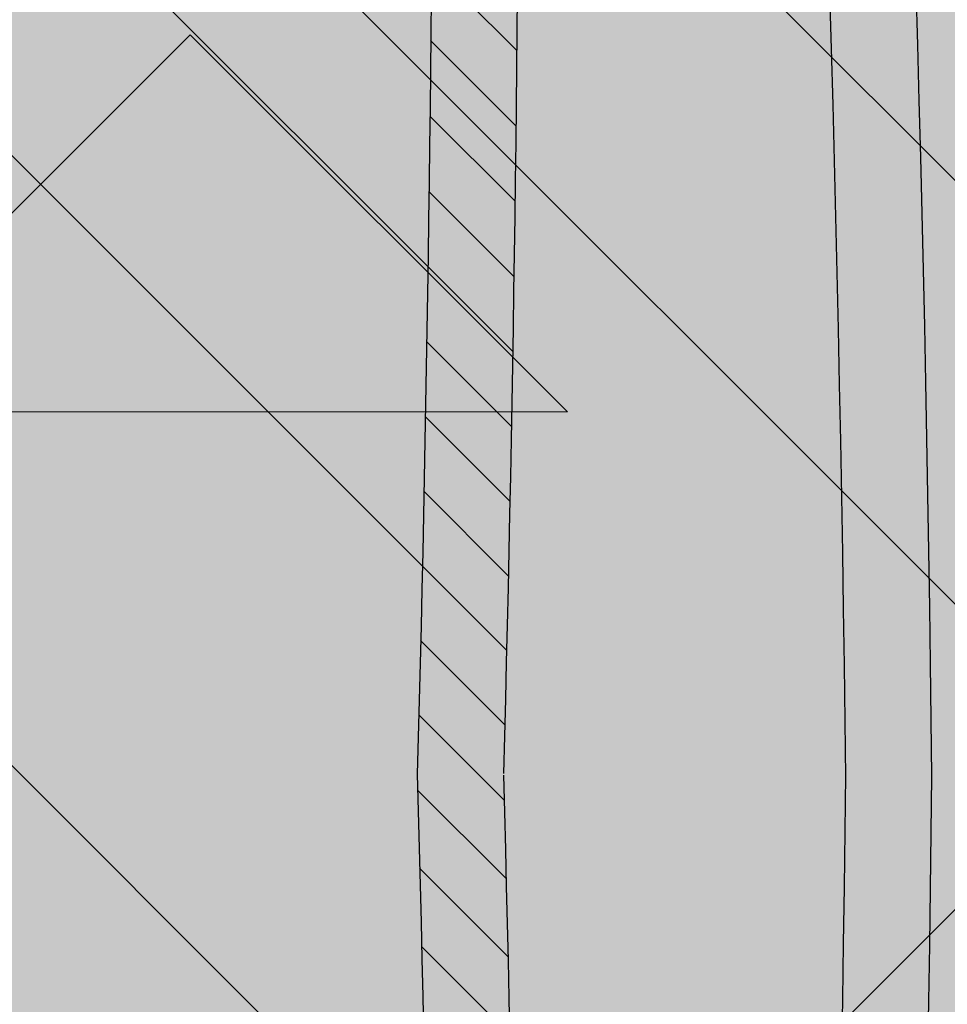
# Model space of a CAD drawing. Units: inches. Extents: x 844 to 2234, y 346 to 1084.
# Tile 34 of 93: x 1260.074 to 1261.788, y 695.763 to 697.583. Entities that reach past the tile are written whole.
import ezdxf

# ---------------------------------------------------------------- set-up
doc = ezdxf.new("R2010")
doc.units = ezdxf.units.IN
doc.header["$MEASUREMENT"] = 0
doc.layers.add('furniture', color=8, linetype='Continuous', lineweight=18)
doc.layers.add('RA-AP-01$0$INT', color=35, linetype='Continuous', lineweight=5)
doc.layers.add('RA-AP-01$0$FURN', color=3, linetype='Continuous')
doc.layers.add('RA-AP-01$0$WOOD', color=64, linetype='Continuous')

# ---------------------------------------------------------------- blocks, each defined once
blk = doc.blocks.new('A$C18D01794')
at = {"layer": 'RA-AP-01$0$INT'}
h = blk.add_hatch(color=256, dxfattribs=at)
h.paths.add_polyline_path([(4.58592, -6.35671), (4.55521, -6.35671), (4.55521, -6.38742), (4.8745, -6.70671), (4.90521, -6.676)])
h.paths.add_polyline_path([(5.25521, -6.38742), (5.25521, -6.35671), (5.2245, -6.35671), (4.90521, -6.676), (4.93592, -6.70671)])
h.paths.add_polyline_path([(4.93592, -6.70671), (4.90521, -6.73742), (5.25521, -7.08742), (5.25521, -7.026)])
h.paths.add_polyline_path([(4.55521, -7.026), (4.55521, -7.08742), (4.90521, -6.73742), (4.8745, -6.70671)])
h = blk.add_hatch(color=256, dxfattribs=at)
h.paths.add_polyline_path([(4.58592, -6.35671), (4.6142, -6.35671), (4.66885, -6.41136), (4.72349, -6.35671), (4.77177, -6.35671), (4.82642, -6.41136), (4.86278, -6.375), (4.8445, -6.35671), (4.86278, -6.35671), (4.90521, -6.39914), (4.94763, -6.35671), (4.96592, -6.35671), (4.94763, -6.375), (4.98399, -6.41136), (5.03864, -6.35671), (5.08692, -6.35671), (5.14157, -6.41136), (5.19621, -6.35671), (5.2245, -6.35671), (4.90521, -6.676)])
h.paths.add_polyline_path([(4.89521, -6.63772), (4.89521, -6.52843), (4.84056, -6.58307)], flags=16)
h.paths.add_polyline_path([(4.91521, -6.63772), (4.96985, -6.58307), (4.91521, -6.52843)], flags=16)
h.paths.add_polyline_path([(4.82642, -6.56893), (4.88106, -6.51429), (4.77177, -6.51429)], flags=16)
h.paths.add_polyline_path([(4.98399, -6.56893), (5.03864, -6.51429), (4.92935, -6.51429)], flags=16)
h.paths.add_polyline_path([(4.88106, -6.49429), (4.82642, -6.43964), (4.77177, -6.49429)], flags=16)
h.paths.add_polyline_path([(4.92935, -6.49429), (5.03864, -6.49429), (4.98399, -6.43964)], flags=16)
h.paths.add_polyline_path([(4.89521, -6.48014), (4.89521, -6.40742), (4.87692, -6.38914), (4.84056, -6.4255)], flags=16)
h.paths.add_polyline_path([(4.91521, -6.48014), (4.96985, -6.4255), (4.93349, -6.38914), (4.91521, -6.40742)], flags=16)
h.paths.add_polyline_path([(4.75763, -6.48014), (4.81228, -6.4255), (4.75763, -6.37085)], flags=16)
h.paths.add_polyline_path([(4.73763, -6.48014), (4.73763, -6.37085), (4.68299, -6.4255)], flags=16)
h.paths.add_polyline_path([(5.05278, -6.48014), (5.05278, -6.37085), (4.99814, -6.4255)], flags=16)
h.paths.add_polyline_path([(5.07278, -6.48014), (5.12742, -6.4255), (5.07278, -6.37085)], flags=16)
h.paths.add_polyline_path([(4.93592, -6.70671), (5.25521, -6.38742), (5.25521, -6.41571), (5.20056, -6.47035), (5.25521, -6.525), (5.25521, -6.57328), (5.20056, -6.62793), (5.23692, -6.66429), (5.25521, -6.646), (5.25521, -6.66429), (5.21278, -6.70671), (5.25521, -6.74914), (5.25521, -6.76742), (5.23692, -6.74914), (5.20056, -6.7855), (5.25521, -6.84014), (5.25521, -6.88843), (5.20056, -6.94307), (5.25521, -6.99772), (5.25521, -7.026)])
h.paths.add_polyline_path([(5.04299, -6.7855), (5.09763, -6.84014), (5.09763, -6.73085)], flags=16)
h.paths.add_polyline_path([(5.02885, -6.77136), (5.08349, -6.71671), (4.9742, -6.71671)], flags=16)
h.paths.add_polyline_path([(5.11763, -6.84014), (5.17228, -6.7855), (5.11763, -6.73085)], flags=16)
h.paths.add_polyline_path([(5.08349, -6.69671), (5.02885, -6.64207), (4.9742, -6.69671)], flags=16)
h.paths.add_polyline_path([(5.13177, -6.85429), (5.18642, -6.79964), (5.24106, -6.85429)], flags=17)
h.paths.add_polyline_path([(5.13177, -6.71671), (5.18642, -6.77136), (5.22278, -6.735), (5.2045, -6.71671)], flags=16)
h.paths.add_polyline_path([(5.09763, -6.68257), (5.09763, -6.57328), (5.04299, -6.62793)], flags=16)
h.paths.add_polyline_path([(5.13177, -6.87429), (5.24106, -6.87429), (5.18642, -6.92893)], flags=17)
h.paths.add_polyline_path([(5.13177, -6.69671), (5.2045, -6.69671), (5.22278, -6.67843), (5.18642, -6.64207)], flags=16)
h.paths.add_polyline_path([(5.11763, -6.68257), (5.17228, -6.62793), (5.11763, -6.57328)], flags=16)
h.paths.add_polyline_path([(5.18642, -6.61378), (5.24106, -6.55914), (5.13177, -6.55914)], flags=16)
h.paths.add_polyline_path([(5.13177, -6.53914), (5.24106, -6.53914), (5.18642, -6.48449)], flags=16)
h.paths.add_polyline_path([(5.25521, -7.08742), (5.25521, -7.10671), (4.55521, -7.10671), (4.55521, -7.08742), (4.90521, -6.73742)])
h.paths.add_polyline_path([(4.98399, -6.84449), (4.92935, -6.89914), (5.03864, -6.89914)], flags=16)
h.paths.add_polyline_path([(4.96985, -6.83035), (4.91521, -6.77571), (4.91521, -6.885)], flags=16)
h.paths.add_polyline_path([(4.92935, -6.91914), (4.98399, -6.97378), (5.03864, -6.91914)], flags=16)
h.paths.add_polyline_path([(5.05278, -6.93328), (4.99814, -6.98793), (5.05278, -7.04257)], flags=16)
h.paths.add_polyline_path([(5.07278, -6.93328), (5.07278, -7.04257), (5.12742, -6.98793)], flags=16)
h.paths.add_polyline_path([(4.89521, -6.77571), (4.84056, -6.83035), (4.89521, -6.885)], flags=16)
h.paths.add_polyline_path([(4.91521, -6.93328), (4.91521, -7.006), (4.93349, -7.02429), (4.96985, -6.98793)], flags=16)
h.paths.add_polyline_path([(4.88106, -6.89914), (4.82642, -6.84449), (4.77177, -6.89914)], flags=16)
h.paths.add_polyline_path([(4.89521, -6.93328), (4.84056, -6.98793), (4.87692, -7.02429), (4.89521, -7.006)], flags=16)
h.paths.add_polyline_path([(4.98399, -7.00207), (4.94763, -7.03843), (4.96592, -7.05671), (5.03864, -7.05671)], flags=16)
h.paths.add_polyline_path([(4.88106, -6.91914), (4.77177, -6.91914), (4.82642, -6.97378)], flags=16)
h.paths.add_polyline_path([(4.90521, -7.01429), (4.86278, -7.05671), (4.94763, -7.05671)], flags=16)
h.paths.add_polyline_path([(5.14157, -7.00207), (5.08692, -7.05671), (5.19621, -7.05671)], flags=16)
h.paths.add_polyline_path([(4.82642, -7.00207), (4.77177, -7.05671), (4.8445, -7.05671), (4.86278, -7.03843)], flags=16)
h.paths.add_polyline_path([(4.81228, -6.98793), (4.75763, -6.93328), (4.75763, -7.04257)], flags=16)
h.paths.add_polyline_path([(4.73763, -6.93328), (4.68299, -6.98793), (4.73763, -7.04257)], flags=16)
h.paths.add_polyline_path([(4.72349, -7.05671), (4.66885, -7.00207), (4.6142, -7.05671)], flags=16)
h.paths.add_polyline_path([(4.59763, -6.70671), (4.55521, -6.66429), (4.55521, -6.646), (4.57349, -6.66429), (4.60985, -6.62793), (4.55521, -6.57328), (4.55521, -6.525), (4.60985, -6.47035), (4.55521, -6.41571), (4.55521, -6.38742), (4.8745, -6.70671), (4.55521, -7.026), (4.55521, -6.99772), (4.60985, -6.94307), (4.55521, -6.88843), (4.55521, -6.84014), (4.60985, -6.7855), (4.57349, -6.74914), (4.55521, -6.76742), (4.55521, -6.74914)])
h.paths.add_polyline_path([(4.71278, -6.73085), (4.71278, -6.84014), (4.76742, -6.7855)], flags=16)
h.paths.add_polyline_path([(4.72692, -6.71671), (4.78157, -6.77136), (4.83621, -6.71671)], flags=16)
h.paths.add_polyline_path([(4.69278, -6.73085), (4.63814, -6.7855), (4.69278, -6.84014)], flags=16)
h.paths.add_polyline_path([(4.72692, -6.69671), (4.83621, -6.69671), (4.78157, -6.64207)], flags=16)
h.paths.add_polyline_path([(4.67864, -6.71671), (4.60592, -6.71671), (4.58763, -6.735), (4.62399, -6.77136)], flags=16)
h.paths.add_polyline_path([(4.71278, -6.68257), (4.76742, -6.62793), (4.71278, -6.57328)], flags=16)
h.paths.add_polyline_path([(4.67864, -6.69671), (4.62399, -6.64207), (4.58763, -6.67843), (4.60592, -6.69671)], flags=16)
h.paths.add_polyline_path([(4.69278, -6.68257), (4.69278, -6.57328), (4.63814, -6.62793)], flags=16)
h.paths.add_polyline_path([(4.62399, -6.79964), (4.67864, -6.85429), (4.56935, -6.85429)], flags=17)
h.paths.add_polyline_path([(4.62399, -6.61378), (4.67864, -6.55914), (4.56935, -6.55914)], flags=16)
h.paths.add_polyline_path([(4.67864, -6.87429), (4.62399, -6.92893), (4.56935, -6.87429)], flags=17)
h.paths.add_polyline_path([(4.67864, -6.53914), (4.62399, -6.48449), (4.56935, -6.53914)], flags=16)
h = blk.add_hatch(color=256, dxfattribs=at)
h.paths.add_polyline_path([(4.58592, -7.85671), (4.6142, -7.85671), (4.66885, -7.80207), (4.72349, -7.85671), (4.77177, -7.85671), (4.82642, -7.80207), (4.86278, -7.83843), (4.8445, -7.85671), (4.86278, -7.85671), (4.90521, -7.81429), (4.94763, -7.85671), (4.96592, -7.85671), (4.94763, -7.83843), (4.98399, -7.80207), (5.03864, -7.85671), (5.08692, -7.85671), (5.14157, -7.80207), (5.19621, -7.85671), (5.2245, -7.85671), (4.90521, -7.53742)])
h.paths.add_polyline_path([(4.89521, -7.57571), (4.89521, -7.685), (4.84056, -7.63035)], flags=16)
h.paths.add_polyline_path([(4.91521, -7.57571), (4.96985, -7.63035), (4.91521, -7.685)], flags=16)
h.paths.add_polyline_path([(4.82642, -7.64449), (4.88106, -7.69914), (4.77177, -7.69914)], flags=16)
h.paths.add_polyline_path([(4.98399, -7.64449), (5.03864, -7.69914), (4.92935, -7.69914)], flags=16)
h.paths.add_polyline_path([(4.88106, -7.71914), (4.82642, -7.77378), (4.77177, -7.71914)], flags=16)
h.paths.add_polyline_path([(4.92935, -7.71914), (5.03864, -7.71914), (4.98399, -7.77378)], flags=16)
h.paths.add_polyline_path([(4.89521, -7.73328), (4.89521, -7.806), (4.87692, -7.82429), (4.84056, -7.78793)], flags=16)
h.paths.add_polyline_path([(4.91521, -7.73328), (4.96985, -7.78793), (4.93349, -7.82429), (4.91521, -7.806)], flags=16)
h.paths.add_polyline_path([(4.75763, -7.73328), (4.81228, -7.78793), (4.75763, -7.84257)], flags=16)
h.paths.add_polyline_path([(4.73763, -7.73328), (4.73763, -7.84257), (4.68299, -7.78793)], flags=16)
h.paths.add_polyline_path([(5.05278, -7.73328), (5.05278, -7.84257), (4.99814, -7.78793)], flags=16)
h.paths.add_polyline_path([(5.07278, -7.73328), (5.12742, -7.78793), (5.07278, -7.84257)], flags=16)
h.paths.add_polyline_path([(4.93592, -7.50671), (5.25521, -7.826), (5.25521, -7.79772), (5.20056, -7.74307), (5.25521, -7.68843), (5.25521, -7.64014), (5.20056, -7.5855), (5.23692, -7.54914), (5.25521, -7.56742), (5.25521, -7.54914), (5.21278, -7.50671), (5.25521, -7.46429), (5.25521, -7.446), (5.23692, -7.46429), (5.20056, -7.42793), (5.25521, -7.37328), (5.25521, -7.325), (5.20056, -7.27035), (5.25521, -7.21571), (5.25521, -7.18742)])
h.paths.add_polyline_path([(5.04299, -7.42793), (5.09763, -7.37328), (5.09763, -7.48257)], flags=16)
h.paths.add_polyline_path([(5.02885, -7.44207), (5.08349, -7.49671), (4.9742, -7.49671)], flags=16)
h.paths.add_polyline_path([(5.11763, -7.37328), (5.17228, -7.42793), (5.11763, -7.48257)], flags=16)
h.paths.add_polyline_path([(5.08349, -7.51671), (5.02885, -7.57136), (4.9742, -7.51671)], flags=16)
h.paths.add_polyline_path([(5.13177, -7.35914), (5.18642, -7.41378), (5.24106, -7.35914)], flags=17)
h.paths.add_polyline_path([(5.13177, -7.49671), (5.18642, -7.44207), (5.22278, -7.47843), (5.2045, -7.49671)], flags=16)
h.paths.add_polyline_path([(5.09763, -7.53085), (5.09763, -7.64014), (5.04299, -7.5855)], flags=16)
h.paths.add_polyline_path([(5.13177, -7.33914), (5.24106, -7.33914), (5.18642, -7.28449)], flags=17)
h.paths.add_polyline_path([(5.13177, -7.51671), (5.2045, -7.51671), (5.22278, -7.535), (5.18642, -7.57136)], flags=16)
h.paths.add_polyline_path([(5.11763, -7.53085), (5.17228, -7.5855), (5.11763, -7.64014)], flags=16)
h.paths.add_polyline_path([(5.18642, -7.59964), (5.24106, -7.65429), (5.13177, -7.65429)], flags=16)
h.paths.add_polyline_path([(5.13177, -7.67429), (5.24106, -7.67429), (5.18642, -7.72893)], flags=16)
h.paths.add_polyline_path([(5.25521, -7.126), (5.25521, -7.10671), (4.55521, -7.10671), (4.55521, -7.126), (4.90521, -7.476)])
h.paths.add_polyline_path([(4.98399, -7.36893), (4.92935, -7.31429), (5.03864, -7.31429)], flags=16)
h.paths.add_polyline_path([(4.96985, -7.38307), (4.91521, -7.43772), (4.91521, -7.32843)], flags=16)
h.paths.add_polyline_path([(4.92935, -7.29429), (4.98399, -7.23964), (5.03864, -7.29429)], flags=16)
h.paths.add_polyline_path([(5.05278, -7.28014), (4.99814, -7.2255), (5.05278, -7.17085)], flags=16)
h.paths.add_polyline_path([(5.07278, -7.28014), (5.07278, -7.17085), (5.12742, -7.2255)], flags=16)
h.paths.add_polyline_path([(4.89521, -7.43772), (4.84056, -7.38307), (4.89521, -7.32843)], flags=16)
h.paths.add_polyline_path([(4.91521, -7.28014), (4.91521, -7.20742), (4.93349, -7.18914), (4.96985, -7.2255)], flags=16)
h.paths.add_polyline_path([(4.88106, -7.31429), (4.82642, -7.36893), (4.77177, -7.31429)], flags=16)
h.paths.add_polyline_path([(4.89521, -7.28014), (4.84056, -7.2255), (4.87692, -7.18914), (4.89521, -7.20742)], flags=16)
h.paths.add_polyline_path([(4.98399, -7.21136), (4.94763, -7.175), (4.96592, -7.15671), (5.03864, -7.15671)], flags=16)
h.paths.add_polyline_path([(4.88106, -7.29429), (4.77177, -7.29429), (4.82642, -7.23964)], flags=16)
h.paths.add_polyline_path([(4.90521, -7.19914), (4.86278, -7.15671), (4.94763, -7.15671)], flags=16)
h.paths.add_polyline_path([(5.14157, -7.21136), (5.08692, -7.15671), (5.19621, -7.15671)], flags=16)
h.paths.add_polyline_path([(4.82642, -7.21136), (4.77177, -7.15671), (4.8445, -7.15671), (4.86278, -7.175)], flags=16)
h.paths.add_polyline_path([(4.81228, -7.2255), (4.75763, -7.28014), (4.75763, -7.17085)], flags=16)
h.paths.add_polyline_path([(4.73763, -7.28014), (4.68299, -7.2255), (4.73763, -7.17085)], flags=16)
h.paths.add_polyline_path([(4.72349, -7.15671), (4.66885, -7.21136), (4.6142, -7.15671)], flags=16)
h.paths.add_polyline_path([(4.59763, -7.50671), (4.55521, -7.54914), (4.55521, -7.56742), (4.57349, -7.54914), (4.60985, -7.5855), (4.55521, -7.64014), (4.55521, -7.68843), (4.60985, -7.74307), (4.55521, -7.79772), (4.55521, -7.826), (4.8745, -7.50671), (4.55521, -7.18742), (4.55521, -7.21571), (4.60985, -7.27035), (4.55521, -7.325), (4.55521, -7.37328), (4.60985, -7.42793), (4.57349, -7.46429), (4.55521, -7.446), (4.55521, -7.46429)])
h.paths.add_polyline_path([(4.71278, -7.48257), (4.71278, -7.37328), (4.76742, -7.42793)], flags=16)
h.paths.add_polyline_path([(4.72692, -7.49671), (4.78157, -7.44207), (4.83621, -7.49671)], flags=16)
h.paths.add_polyline_path([(4.69278, -7.48257), (4.63814, -7.42793), (4.69278, -7.37328)], flags=16)
h.paths.add_polyline_path([(4.72692, -7.51671), (4.83621, -7.51671), (4.78157, -7.57136)], flags=16)
h.paths.add_polyline_path([(4.67864, -7.49671), (4.60592, -7.49671), (4.58763, -7.47843), (4.62399, -7.44207)], flags=16)
h.paths.add_polyline_path([(4.71278, -7.53085), (4.76742, -7.5855), (4.71278, -7.64014)], flags=16)
h.paths.add_polyline_path([(4.67864, -7.51671), (4.62399, -7.57136), (4.58763, -7.535), (4.60592, -7.51671)], flags=16)
h.paths.add_polyline_path([(4.69278, -7.53085), (4.69278, -7.64014), (4.63814, -7.5855)], flags=16)
h.paths.add_polyline_path([(4.62399, -7.41378), (4.67864, -7.35914), (4.56935, -7.35914)], flags=17)
h.paths.add_polyline_path([(4.62399, -7.59964), (4.67864, -7.65429), (4.56935, -7.65429)], flags=16)
h.paths.add_polyline_path([(4.67864, -7.33914), (4.62399, -7.28449), (4.56935, -7.33914)], flags=17)
h.paths.add_polyline_path([(4.67864, -7.67429), (4.62399, -7.72893), (4.56935, -7.67429)], flags=16)
h = blk.add_hatch(color=256, dxfattribs=at)
h.paths.add_polyline_path([(4.90521, -7.53742), (4.8745, -7.50671), (4.55521, -7.826), (4.55521, -7.85671), (4.58592, -7.85671)])
h.paths.add_polyline_path([(4.93592, -7.50671), (4.90521, -7.53742), (5.2245, -7.85671), (5.25521, -7.85671), (5.25521, -7.826)])
h.paths.add_polyline_path([(5.25521, -7.18742), (5.25521, -7.126), (4.90521, -7.476), (4.93592, -7.50671)])
h.paths.add_polyline_path([(4.8745, -7.50671), (4.90521, -7.476), (4.55521, -7.126), (4.55521, -7.18742)])
h = blk.add_hatch(color=256, dxfattribs=at)
h.paths.add_polyline_path([(4.89521, -7.32843), (4.84056, -7.38307), (4.89521, -7.43772)])
h.paths.add_polyline_path([(4.91521, -7.43772), (4.96985, -7.38307), (4.91521, -7.32843)])
h.paths.add_polyline_path([(4.92935, -7.31429), (4.98399, -7.36893), (5.03864, -7.31429)])
h.paths.add_polyline_path([(5.03864, -7.29429), (4.98399, -7.23964), (4.92935, -7.29429)])
h.paths.add_polyline_path([(4.96985, -7.2255), (4.93349, -7.18914), (4.91521, -7.20742), (4.91521, -7.28014)])
h.paths.add_polyline_path([(4.96592, -7.15671), (4.94763, -7.175), (4.98399, -7.21136), (5.03864, -7.15671)])
h.paths.add_polyline_path([(4.99814, -7.2255), (5.05278, -7.28014), (5.05278, -7.17085)])
h.paths.add_polyline_path([(5.07278, -7.28014), (5.12742, -7.2255), (5.07278, -7.17085)])
h.paths.add_polyline_path([(5.19621, -7.15671), (5.08692, -7.15671), (5.14157, -7.21136)])
h.paths.add_polyline_path([(4.86278, -7.15671), (4.90521, -7.19914), (4.94763, -7.15671)])
h.paths.add_polyline_path([(4.89521, -7.28014), (4.89521, -7.20742), (4.87692, -7.18914), (4.84056, -7.2255)])
h.paths.add_polyline_path([(4.82642, -7.23964), (4.77177, -7.29429), (4.88106, -7.29429)])
h.paths.add_polyline_path([(4.77177, -7.31429), (4.82642, -7.36893), (4.88106, -7.31429)])
h.paths.add_polyline_path([(4.75763, -7.28014), (4.81228, -7.2255), (4.75763, -7.17085)])
h.paths.add_polyline_path([(4.86278, -7.175), (4.8445, -7.15671), (4.77177, -7.15671), (4.82642, -7.21136)])
h.paths.add_polyline_path([(4.68299, -7.2255), (4.73763, -7.28014), (4.73763, -7.17085)])
h.paths.add_polyline_path([(4.72349, -7.15671), (4.6142, -7.15671), (4.66885, -7.21136)])
for p, q in [((4.90521, -6.73742), (4.55521, -7.08742)), ((4.90521, -7.476), (4.55521, -7.126)), ((4.72349, -7.15671), (4.6142, -7.15671)), ((4.6142, -7.15671), (4.66885, -7.21136)), ((4.72349, -7.15671), (4.66885, -7.21136)), ((4.8745, -7.50671), (4.55521, -7.18742))]:
    blk.add_line(p, q, dxfattribs=at)
blk = doc.blocks.new('A$C32926AE1')
at = {"layer": 'RA-AP-01$0$WOOD'}
h = blk.add_hatch(color=256, dxfattribs=at)
h.dxf.hatch_style = 1
h.paths.add_polyline_path([(5.15743, 4.57348, -0.100949), (5.1554, 4.59337, -0.184266), (5.17225, 4.6388, 0.205661), (5.17956, 4.66132, 0.361434), (5.13435, 4.70652, 0.205661), (5.11183, 4.69921, -0.184266), (5.0664, 4.68237, -0.105531), (5.04566, 4.68467, 0.156764), (4.76389, 4.68467, -0.105531), (4.74314, 4.68237, -0.184266), (4.69771, 4.69921, 0.205661), (4.67519, 4.70652, 0.361434), (4.62998, 4.66132, 0.205661), (4.63729, 4.6388, -0.184266), (4.65414, 4.59337, -0.100949), (4.65211, 4.57348, 0.02141), (4.62975, 4.15671, 0.02141), (4.65211, 3.73994, -0.100949), (4.65414, 3.72006, -0.184266), (4.63729, 3.67463, 0.205661), (4.62998, 3.65211, 0.361434), (4.67519, 3.6069, 0.205661), (4.69771, 3.61421, -0.184266), (4.74314, 3.63106, -0.105531), (4.76389, 3.62875, 0.156764), (5.04566, 3.62875, -0.105531), (5.0664, 3.63106, -0.184266), (5.11183, 3.61421, 0.205661), (5.13435, 3.6069, 0.361434), (5.17956, 3.65211, 0.205661), (5.17225, 3.67463, -0.184266), (5.1554, 3.72006, -0.100949), (5.15743, 3.73994, 0.02141), (5.17979, 4.15671, 0.02141)])
h.paths.add_polyline_path([(4.63975, 4.15671, 0.021354), (4.66197, 3.74189, -0.094076), (4.66414, 3.71961, -0.182482), (4.64481, 3.66804, 0.205661), (4.63994, 3.65302, 0.361434), (4.67611, 3.61686, 0.205661), (4.69112, 3.62173, -0.182482), (4.7427, 3.64106, -0.102989), (4.76699, 3.63826, 0.156709), (5.04255, 3.63826, -0.102989), (5.06685, 3.64106, -0.182482), (5.11842, 3.62173, 0.205661), (5.13344, 3.61686, 0.361434), (5.1696, 3.65302, 0.205661), (5.16473, 3.66804, -0.182482), (5.1454, 3.71961, -0.094076), (5.14757, 3.74189, 0.021354), (5.16979, 4.15671, 0.021354), (5.14757, 4.57154, -0.094076), (5.1454, 4.59381, -0.182482), (5.16473, 4.64539, 0.205661), (5.1696, 4.6604, 0.361434), (5.13344, 4.69657, 0.205661), (5.11842, 4.69169, -0.182482), (5.06685, 4.67236, -0.102989), (5.04255, 4.67517, 0.156709), (4.76699, 4.67517, -0.102989), (4.7427, 4.67236, -0.182482), (4.69112, 4.69169, 0.205661), (4.67611, 4.69657, 0.361434), (4.63994, 4.6604, 0.205661), (4.64481, 4.64539, -0.182482), (4.66414, 4.59381, -0.094076), (4.66197, 4.57154, 0.021354)], flags=16)
h.paths.add_polyline_path([(5.12979, 4.43217, -0.014166), (5.13015, 4.15693, -0.014166), (5.12979, 3.88169, -0.078525), (5.1098, 3.75514, 0.094597), (5.10541, 3.7179, 0.104317), (5.11607, 3.67039, 0.104317), (5.06856, 3.68105, 0.094597), (5.03132, 3.67666, -0.158024), (4.77823, 3.67666, 0.094597), (4.74098, 3.68105, 0.104317), (4.69347, 3.67039, 0.104317), (4.70413, 3.7179, 0.094597), (4.69975, 3.75514, -0.078525), (4.67975, 3.88169, -0.014166), (4.67939, 4.15693, -0.014166), (4.67975, 4.43217, -0.078525), (4.69975, 4.55871, 0.094597), (4.70413, 4.59596, 0.104317), (4.69347, 4.64347, 0.104317), (4.74098, 4.6328, 0.094597), (4.77823, 4.63719, -0.158024), (5.03132, 4.63719, 0.094597), (5.06856, 4.6328, 0.104317), (5.11607, 4.64347, 0.104317), (5.10541, 4.59596, 0.094597), (5.1098, 4.55871, -0.078525)], flags=0)
h.paths.add_polyline_path([(5.11979, 4.43226, -0.0142), (5.12016, 4.15693, -0.0142), (5.11979, 3.8816, -0.078489), (5.10027, 3.75819, 0.094014), (5.09541, 3.71748, 0.060627), (5.09962, 3.68684, 0.060627), (5.06898, 3.69105, 0.094014), (5.02827, 3.68619, -0.158071), (4.78127, 3.68619, 0.094014), (4.74056, 3.69105, 0.060627), (4.70993, 3.68684, 0.060627), (4.71413, 3.71748, 0.094014), (4.70927, 3.75819, -0.078489), (4.68975, 3.8816, -0.0142), (4.68939, 4.15693, -0.0142), (4.68975, 4.43226, -0.078489), (4.70927, 4.55566, 0.094014), (4.71413, 4.59638, 0.060627), (4.70993, 4.62701, 0.060627), (4.74056, 4.62281, 0.094014), (4.78127, 4.62767, -0.158071), (5.02827, 4.62767, 0.094014), (5.06898, 4.62281, 0.060627), (5.09962, 4.62701, 0.060627), (5.09541, 4.59638, 0.094014), (5.10027, 4.55566, -0.078489)], flags=0)
h.paths.add_polyline_path([(5.06979, 4.43022, -0.014242), (5.07017, 4.15693, -0.014242), (5.06979, 3.88364, -0.080061), (5.05266, 3.77346, 0.052642), (5.04591, 3.74055, 0.052642), (5.013, 3.7338, -0.158303), (4.79655, 3.7338, 0.052642), (4.76363, 3.74055, 0.052642), (4.75688, 3.77346, -0.080061), (4.73975, 3.88364, -0.014242), (4.73937, 4.15693, -0.014242), (4.73975, 4.43022, -0.080061), (4.75688, 4.54039, 0.052642), (4.76363, 4.5733, 0.052642), (4.79655, 4.58006, -0.158303), (5.013, 4.58006, 0.052642), (5.04591, 4.5733, 0.052642), (5.05266, 4.54039, -0.080061)], flags=0)
h.paths.add_polyline_path([(5.04979, 4.43038, -0.01431), (5.05018, 4.15693, -0.01431), (5.04979, 3.88347, -0.080069), (5.03362, 3.77958, 0.030626), (5.02824, 3.75822, 0.030626), (5.00688, 3.75284, -0.158398), (4.80266, 3.75284, 0.030626), (4.7813, 3.75822, 0.030626), (4.77592, 3.77958, -0.080069), (4.75975, 3.88347, -0.01431), (4.75936, 4.15693, -0.01431), (4.75975, 4.43038, -0.080069), (4.77592, 4.53427, 0.030626), (4.7813, 4.55564, 0.030626), (4.80266, 4.56102, -0.158398), (5.00688, 4.56102, 0.030626), (5.02824, 4.55564, 0.030626), (5.03362, 4.53427, -0.080069)], flags=0)
h.paths.add_polyline_path([(4.99977, 4.42817, -0.014344), (5.0002, 4.15693, -0.014344), (4.99977, 3.88568, -0.078464), (4.98736, 3.7991, -0.150605), (4.82219, 3.7991, -0.078464), (4.80978, 3.88568, -0.014344), (4.80934, 4.15693, -0.014344), (4.80978, 4.42817, -0.078464), (4.82219, 4.51475, -0.150605), (4.98736, 4.51475, -0.078464)], flags=0)
h.paths.add_polyline_path([(4.97976, 4.42764, -0.014377), (4.98021, 4.15693, -0.014377), (4.97976, 3.88621, -0.068924), (4.97118, 3.81528, -0.129665), (4.83836, 3.81528, -0.068924), (4.82979, 3.88621, -0.014377), (4.82934, 4.15693, -0.014377), (4.82979, 4.42764, -0.068924), (4.83836, 4.49858, -0.129665), (4.97118, 4.49858, -0.068924)], flags=0)
h = blk.add_hatch(color=256, dxfattribs=at)
h.dxf.hatch_style = 1
h.paths.add_polyline_path([(5.1454, 4.59381, -0.182482), (5.16473, 4.64539, 0.205661), (5.1696, 4.6604, 0.361434), (5.13344, 4.69657, 0.205661), (5.11842, 4.69169, -0.182482), (5.06685, 4.67236, -0.102989), (5.04255, 4.67517, 0.156709), (4.76699, 4.67517, -0.102989), (4.7427, 4.67236, -0.182482), (4.69112, 4.69169, 0.205661), (4.67611, 4.69657, 0.361434), (4.63994, 4.6604, 0.205661), (4.64481, 4.64539, -0.182482), (4.66414, 4.59381, -0.094076), (4.66197, 4.57154, 0.021354), (4.63975, 4.15671, 0.021354), (4.66197, 3.74189, -0.094076), (4.66414, 3.71961, -0.182482), (4.64481, 3.66804, 0.205661), (4.63994, 3.65302, 0.361434), (4.67611, 3.61686, 0.205661), (4.69112, 3.62173, -0.182482), (4.7427, 3.64106, -0.102989), (4.76699, 3.63826, 0.156709), (5.04255, 3.63826, -0.102989), (5.06685, 3.64106, -0.182482), (5.11842, 3.62173, 0.205661), (5.13344, 3.61686, 0.361434), (5.1696, 3.65302, 0.205661), (5.16473, 3.66804, -0.182482), (5.1454, 3.71961, -0.094076), (5.14757, 3.74189, 0.021354), (5.16979, 4.15671, 0.021354), (5.14757, 4.57154, -0.094076)])
h.paths.add_polyline_path([(5.1098, 4.55871, -0.078525), (5.12979, 4.43217, -0.014166), (5.13015, 4.15693, -0.014166), (5.12979, 3.88169, -0.078525), (5.1098, 3.75514, 0.094597), (5.10541, 3.7179, 0.104317), (5.11607, 3.67039, 0.104317), (5.06856, 3.68105, 0.094597), (5.03132, 3.67666, -0.158024), (4.77823, 3.67666, 0.094597), (4.74098, 3.68105, 0.104317), (4.69347, 3.67039, 0.104317), (4.70413, 3.7179, 0.094597), (4.69975, 3.75514, -0.078525), (4.67975, 3.88169, -0.014166), (4.67939, 4.15693, -0.014166), (4.67975, 4.43217, -0.078525), (4.69975, 4.55871, 0.094597), (4.70413, 4.59596, 0.104317), (4.69347, 4.64347, 0.104317), (4.74098, 4.6328, 0.094597), (4.77823, 4.63719, -0.158024), (5.03132, 4.63719, 0.094597), (5.06856, 4.6328, 0.104317), (5.11607, 4.64347, 0.104317), (5.10541, 4.59596, 0.094597)], flags=16)
h.paths.add_polyline_path([(5.10027, 4.55566, -0.078489), (5.11979, 4.43226, -0.0142), (5.12016, 4.15693, -0.0142), (5.11979, 3.8816, -0.078489), (5.10027, 3.75819, 0.094014), (5.09541, 3.71748, 0.060627), (5.09962, 3.68684, 0.060627), (5.06898, 3.69105, 0.094014), (5.02827, 3.68619, -0.158071), (4.78127, 3.68619, 0.094014), (4.74056, 3.69105, 0.060627), (4.70993, 3.68684, 0.060627), (4.71413, 3.71748, 0.094014), (4.70927, 3.75819, -0.078489), (4.68975, 3.8816, -0.0142), (4.68939, 4.15693, -0.0142), (4.68975, 4.43226, -0.078489), (4.70927, 4.55566, 0.094014), (4.71413, 4.59638, 0.060627), (4.70993, 4.62701, 0.060627), (4.74056, 4.62281, 0.094014), (4.78127, 4.62767, -0.158071), (5.02827, 4.62767, 0.094014), (5.06898, 4.62281, 0.060627), (5.09962, 4.62701, 0.060627), (5.09541, 4.59638, 0.094014)], flags=0)
h.paths.add_polyline_path([(5.04591, 4.5733, 0.052642), (5.05266, 4.54039, -0.080061), (5.06979, 4.43022, -0.014242), (5.07017, 4.15693, -0.014242), (5.06979, 3.88364, -0.080061), (5.05266, 3.77346, 0.052642), (5.04591, 3.74055, 0.052642), (5.013, 3.7338, -0.158303), (4.79655, 3.7338, 0.052642), (4.76363, 3.74055, 0.052642), (4.75688, 3.77346, -0.080061), (4.73975, 3.88364, -0.014242), (4.73937, 4.15693, -0.014242), (4.73975, 4.43022, -0.080061), (4.75688, 4.54039, 0.052642), (4.76363, 4.5733, 0.052642), (4.79655, 4.58006, -0.158303), (5.013, 4.58006, 0.052642)], flags=0)
h.paths.add_polyline_path([(5.02824, 4.55564, 0.030626), (5.03362, 4.53427, -0.080069), (5.04979, 4.43038, -0.01431), (5.05018, 4.15693, -0.01431), (5.04979, 3.88347, -0.080069), (5.03362, 3.77958, 0.030626), (5.02824, 3.75822, 0.030626), (5.00688, 3.75284, -0.158398), (4.80266, 3.75284, 0.030626), (4.7813, 3.75822, 0.030626), (4.77592, 3.77958, -0.080069), (4.75975, 3.88347, -0.01431), (4.75936, 4.15693, -0.01431), (4.75975, 4.43038, -0.080069), (4.77592, 4.53427, 0.030626), (4.7813, 4.55564, 0.030626), (4.80266, 4.56102, -0.158398), (5.00688, 4.56102, 0.030626)], flags=0)
h.paths.add_polyline_path([(4.98736, 4.51475, -0.078464), (4.99977, 4.42817, -0.014344), (5.0002, 4.15693, -0.014344), (4.99977, 3.88568, -0.078464), (4.98736, 3.7991, -0.150605), (4.82219, 3.7991, -0.078464), (4.80978, 3.88568, -0.014344), (4.80934, 4.15693, -0.014344), (4.80978, 4.42817, -0.078464), (4.82219, 4.51475, -0.150605)], flags=0)
h.paths.add_polyline_path([(4.97118, 4.49858, -0.068924), (4.97976, 4.42764, -0.014377), (4.98021, 4.15693, -0.014377), (4.97976, 3.88621, -0.068924), (4.97118, 3.81528, -0.129665), (4.83836, 3.81528, -0.068924), (4.82979, 3.88621, -0.014377), (4.82934, 4.15693, -0.014377), (4.82979, 4.42764, -0.068924), (4.83836, 4.49858, -0.129665)], flags=0)
h = blk.add_hatch(dxfattribs=at)
h.set_pattern_fill('ANSI31', color=256, scale=0.05, style=0)
h.paths.add_polyline_path([(5.13015, 4.15693, 0.014166), (5.12979, 4.43217, 0.077783), (5.11017, 4.55756, -0.097652), (5.10541, 4.59596, -0.104317), (5.11607, 4.64347), (5.09962, 4.62701, 0.060627), (5.09541, 4.59638, 0.094014), (5.10027, 4.55566, -0.078489), (5.11979, 4.43226, -0.0142), (5.12016, 4.15693, -0.0142), (5.11979, 3.8816, -0.078489), (5.10027, 3.75819, 0.094014), (5.09541, 3.71748, 0.060627), (5.09962, 3.68684), (5.11607, 3.67039, -0.104317), (5.10541, 3.7179, -0.097652), (5.11017, 3.7563, 0.077783), (5.12979, 3.88169, 0.014166)])
h.paths.add_polyline_path([(5.03016, 3.67629, -0.097652), (5.06856, 3.68105, -0.104317), (5.11607, 3.67039), (5.09962, 3.68684, 0.060627), (5.06898, 3.69105, 0.094014), (5.02827, 3.68619, -0.158071), (4.78127, 3.68619, 0.094014), (4.74056, 3.69105, 0.060627), (4.70993, 3.68684), (4.69347, 3.67039, -0.104317), (4.74098, 3.68105, -0.097652), (4.77938, 3.67629, 0.156513)])
h.paths.add_polyline_path([(4.68975, 3.8816, -0.0142), (4.68939, 4.15693, -0.0142), (4.68975, 4.43226, -0.078489), (4.70927, 4.55566, 0.094014), (4.71413, 4.59638, 0.060627), (4.70993, 4.62701), (4.69347, 4.64347, -0.104317), (4.70413, 4.59596, -0.097652), (4.69937, 4.55756, 0.077783), (4.67975, 4.43217, 0.014166), (4.67939, 4.15693, 0.014166), (4.67975, 3.88169, 0.077783), (4.69937, 3.7563, -0.097652), (4.70413, 3.7179, -0.104317), (4.69347, 3.67039), (4.70993, 3.68684, 0.060627), (4.71413, 3.71748, 0.094014), (4.70927, 3.75819, -0.078489)])
h.paths.add_polyline_path([(4.77938, 4.63756, -0.097652), (4.74098, 4.6328, -0.104317), (4.69347, 4.64347), (4.70993, 4.62701, 0.060627), (4.74056, 4.62281, 0.094014), (4.78127, 4.62767, -0.158071), (5.02827, 4.62767, 0.094014), (5.06898, 4.62281, 0.060627), (5.09962, 4.62701), (5.11607, 4.64347, -0.104317), (5.06856, 4.6328, -0.097652), (5.03016, 4.63756, 0.156513)])
h = blk.add_hatch(dxfattribs=at)
h.set_pattern_fill('ANSI32', color=256, scale=0.2, style=0)
h.paths.add_polyline_path([(5.11979, 4.43226, 0.077702), (5.10066, 4.55447, -0.09689), (5.09541, 4.59638, -0.060627), (5.09962, 4.62701, -0.060627), (5.06898, 4.62281, -0.09689), (5.02707, 4.62805, 0.156466), (4.78247, 4.62805, -0.09689), (4.74056, 4.62281, -0.060627), (4.70993, 4.62701, -0.060627), (4.71413, 4.59638, -0.09689), (4.70888, 4.55447, 0.077702), (4.68975, 4.43226, 0.0142), (4.68939, 4.15693, 0.0142), (4.68975, 3.8816, 0.077702), (4.70888, 3.75939, -0.09689), (4.71413, 3.71748, -0.060627), (4.70993, 3.68684, -0.060627), (4.74056, 3.69105, -0.09689), (4.78247, 3.6858, 0.156466), (5.02707, 3.6858, -0.09689), (5.06898, 3.69105, -0.060627), (5.09962, 3.68684, -0.060627), (5.09541, 3.71748, -0.09689), (5.10066, 3.75939, 0.077702), (5.11979, 3.8816, 0.0142), (5.12016, 4.15693, 0.0142)])
h.paths.add_polyline_path([(5.07017, 4.15693, -0.014242), (5.06979, 3.88364, -0.080061), (5.05266, 3.77346, 0.052642), (5.04591, 3.74055, 0.052642), (5.013, 3.7338, -0.158303), (4.79655, 3.7338, 0.052642), (4.76363, 3.74055, 0.052642), (4.75688, 3.77346, -0.080061), (4.73975, 3.88364, -0.014242), (4.73937, 4.15693, -0.014242), (4.73975, 4.43022, -0.080061), (4.75688, 4.54039, 0.052642), (4.76363, 4.5733, 0.052642), (4.79655, 4.58006, -0.158303), (5.013, 4.58006, 0.052642), (5.04591, 4.5733, 0.052642), (5.05266, 4.54039, -0.080061), (5.06979, 4.43022, -0.014242)], flags=16)
h.paths.add_polyline_path([(5.05018, 4.15693, -0.01431), (5.04979, 3.88347, -0.080069), (5.03362, 3.77958, 0.030626), (5.02824, 3.75822, 0.030626), (5.00688, 3.75284, -0.158398), (4.80266, 3.75284, 0.030626), (4.7813, 3.75822, 0.030626), (4.77592, 3.77958, -0.080069), (4.75975, 3.88347, -0.01431), (4.75936, 4.15693, -0.01431), (4.75975, 4.43038, -0.080069), (4.77592, 4.53427, 0.030626), (4.7813, 4.55564, 0.030626), (4.80266, 4.56102, -0.158398), (5.00688, 4.56102, 0.030626), (5.02824, 4.55564, 0.030626), (5.03362, 4.53427, -0.080069), (5.04979, 4.43038, -0.01431)], flags=0)
h.paths.add_polyline_path([(5.0002, 4.15693, -0.014344), (4.99977, 3.88568, -0.078464), (4.98736, 3.7991, -0.150605), (4.82219, 3.7991, -0.078464), (4.80978, 3.88568, -0.014344), (4.80934, 4.15693, -0.014344), (4.80978, 4.42817, -0.078464), (4.82219, 4.51475, -0.150605), (4.98736, 4.51475, -0.078464), (4.99977, 4.42817, -0.014344)], flags=0)
h.paths.add_polyline_path([(4.98021, 4.15693, -0.014377), (4.97976, 3.88621, -0.068924), (4.97118, 3.81528, -0.129665), (4.83836, 3.81528, -0.068924), (4.82979, 3.88621, -0.014377), (4.82934, 4.15693, -0.014377), (4.82979, 4.42764, -0.068924), (4.83836, 4.49858, -0.129665), (4.97118, 4.49858, -0.068924), (4.97976, 4.42764, -0.014377)], flags=0)
for centre, radius, start, end in [((9.50522, 4.10408), 4.87575, 174.47541, 179.3815), ((9.50522, 4.10408), 4.86575, 174.48704, 179.3815), ((9.53595, 4.28823), 4.85833, 178.30224, 181.54738), ((9.53595, 4.28823), 4.84835, 178.3067, 181.55184), ((9.50522, 4.20934), 4.87575, 180.6185, 185.52459), ((9.50522, 4.20934), 4.86575, 180.6185, 185.51296), ((9.53595, 4.02563), 4.85833, 178.45262, 181.69776), ((9.53595, 4.02563), 4.84835, 178.44816, 181.6933)]:
    blk.add_arc(centre, radius, start, end, dxfattribs=at)
blk = doc.blocks.new('A$C5D2F253E')
at = {"layer": 'RA-AP-01$0$FURN', "xscale": -0.7999999999883585, "yscale": 0.7999999999883585, "zscale": 0.8, "rotation": 90}
blk.add_blockref('A$C18D01794', (-5.68776, 4.75792), dxfattribs=at)
at = {"layer": 'RA-AP-01$0$WOOD', "rotation": 270}
blk.add_blockref('A$C32926AE1', (-4.16134, 5.73853), dxfattribs=at)

msp = doc.modelspace()

# ---------------------------------------------------------------- block references
at = {"layer": 'furniture', "xscale": -15.94108302203742, "yscale": 15.94108302203742, "zscale": 15.94108302203742, "rotation": 270}
msp.add_blockref('A$C5D2F253E', (1244.0841, 696.2585), dxfattribs=at)

doc.saveas('drawing.dxf')
